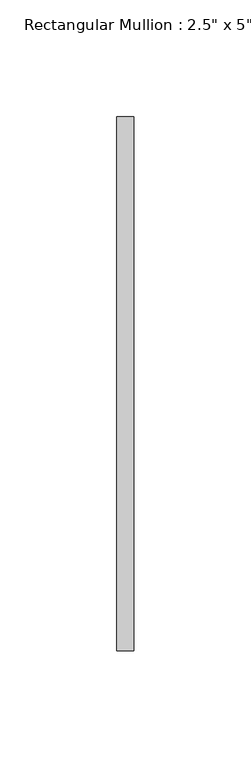
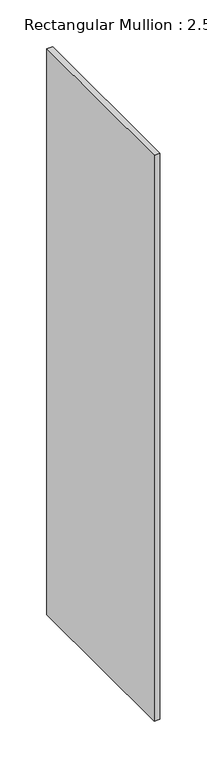
"""IFC4 building model written with IfcOpenShell, lengths in millimetres: member geometry."""

from ifc_helpers import new_model, si_unit, frame, origin, place, context, project, spatial, polyline, outline, extrude, source, transform, mapped, element, save


def member_3448d7e6(model_context):
    return source(origin(), model_context, "Body", "SweptSolid", [
        extrude(outline(polyline([(0.0, 114.3), (0.0, -114.3), (-7.239, -114.3), (-7.239, 114.3), (0.0, 114.3)])), frame((0.0, 0.0, -736.6), z_axis=(0.0, 0.0, 1.0), x_axis=(1.0, 0.0, 0.0)), (0.0, 0.0, 1.0), 736.6),
    ])


if __name__ == "__main__":
    model = new_model("IFC4")
    model_context = context("Model", 3, world=origin())
    ifc_project = project(units=[si_unit("LENGTHUNIT", "METRE", prefix="MILLI")], contexts=[model_context])
    site = spatial("IfcSite", under=ifc_project)
    building = spatial("IfcBuilding", under=site)
    placement = place(None, origin())
    member_shape = member_3448d7e6(model_context)
    element("IfcMember", 1, ObjectType="Rectangular Mullion : 2.5\" x 5\" rectangular", at=placement, inside=building, context=model_context, shape_type="MappedRepresentation", body=[
        mapped(member_shape, transform((0.0, 0.0, 0.0), x_axis=(1.0, 0.0, 0.0), y_axis=(0.0, 1.0, 0.0), z_axis=(0.0, 0.0, 1.0))),
    ])
    save(model, "model.ifc")

# Revit data of these elements
# Type "Rectangular Mullion : 2.5\" x 5\" rectangular"
#   built-in parameter 1007304 = 0.75 (stored number, unit not read)
#   built-in parameter 1007301 = 0.011875 (stored number, unit not read)
#   built-in parameter 1007300 = 0.011875 (stored number, unit not read)
# Element 1 (IfcMember, "Rectangular Mullion : 2.5\" x 5\" rectangular")
#   Materials on its faces: "WINDOW GLASS MATERIAL"
# Materials
#   "WINDOW GLASS MATERIAL": class "Generic", colour RGB 120 120 120, transparency 0, Cost = 0
